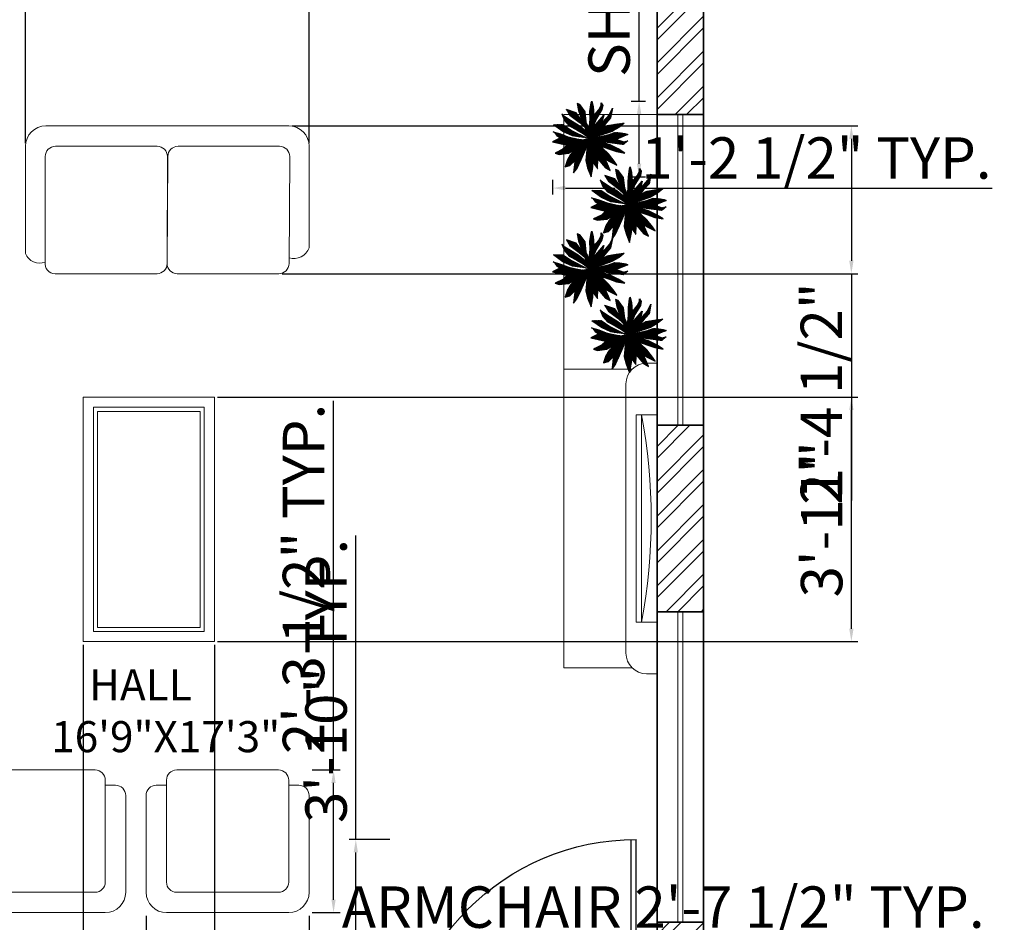
# Model space of a CAD drawing. Units: inches. Extents: x 3595 to 4516, y 2363 to 2965.
# Tile 9 of 12: x 4309 to 4499, y 2512 to 2686. Entities that reach past the tile are written whole.
import ezdxf

# ---------------------------------------------------------------- set-up
doc = ezdxf.new("R2010")
doc.units = ezdxf.units.IN
for name, color, linetype, lineweight in [('A-ANNO-DIMS', 2, 'Continuous', 18), ('A-AREA-IDEN', 7, 'Continuous', 18), ('A-DOOR', 4, 'Continuous', 25), ('A-EQPM', 8, 'Continuous', 18), ('A-FLOR-CASE', 9, 'Continuous', 18), ('A-FURN', 43, 'Continuous', 18), ('A-GLAZ', 4, 'Continuous', 18), ('A-WALL', 7, 'Continuous', 35), ('L-PLNT', 3, 'Continuous', 13), ('vfolhas', 114, 'Continuous', 5)]:
    doc.layers.add(name, color=color, linetype=linetype, lineweight=lineweight)
doc.layers.add('A-WALL-PATT', color=251, linetype='Continuous', lineweight=13, true_color=0x636466)
for name, color, linetype in [('vfolha', 72, 'Continuous'), ('vfolha2', 110, 'Continuous'), ('vfolhas2', 102, 'Continuous')]:
    doc.layers.add(name, color=color, linetype=linetype)
doc.styles.get("Standard").update_dxf_attribs({"font": 'arial.ttf'})
doc.dimstyles.new('ISO-25', dxfattribs={"dimtxt": 8, "dimasz": 2.5, "dimexe": 1.25, "dimexo": 0.625, "dimtad": 1, "dimdec": 1, "dimlunit": 3, "dimtxsty": 'Standard', "dimcen": 2.5, "dimadec": 0, "dimazin": 0, "dimtfac": 1, "dimtdec": 1, "dimtmove": 0, "dimatfit": 3, "dimfxl": 1, "dimarcsym": 0})
pattern_1 = [(45, (-2446.5133113, 50.986076), (-0.004419417382, 0.004419417382), [])]

# ---------------------------------------------------------------- blocks, each defined once
blk = doc.blocks.new('D')
for p, q in [((1, 0), (1, 46)), ((2, 0), (2, 46)), ((0, 0), (2, 0)), ((47, 0), (48, 0))]:
    blk.add_line(p, q)
at = {"ltscale": 0.5}
blk.add_arc((1, 0), 46, 0, 90, dxfattribs=at)
blk = doc.blocks.new('arbusto_PB_verde_grande')
at = {"layer": 'vfolha2'}
h = blk.add_hatch(dxfattribs=at)
h.set_pattern_fill('ANSI31', color=256, scale=0.05, style=0)
h.set_pattern_definition(pattern_1)
h.paths.add_polyline_path([(0.029, 0.357), (0, 0.09), (0.026, -0.039), (0.047, 0.062), (0.062, 0.097), (0.094, 0.266), (0.1, 0.435), (0.088, 0.613), (0.064, 0.723), (0.05, 0.685), (0.024, 0.513)])
h.paths.add_polyline_path([(0.301, 0.438), (0.142, 0.249), (0.267, 0.3)])
h.paths.add_polyline_path([(0.38, 0.228), (0.237, 0.152), (0.184, 0.094), (0.111, 0.044), (0.026, -0.039), (0.281, 0.047), (0.368, 0.078), (0.468, 0.112), (0.611, 0.194), (0.716, 0.278), (0.558, 0.259)])
h.paths.add_polyline_path([(0.561, -0.294), (0.728, -0.326), (0.59, -0.241), (0.43, -0.16), (0.026, -0.039), (0.149, -0.141), (0.188, -0.166), (0.415, -0.244)])
h.paths.add_polyline_path([(-0.274, -0.448), (-0.304, -0.726), (-0.239, -0.642), (-0.155, -0.457), (0.026, -0.039), (-0.163, -0.254)])
h.paths.add_polyline_path([(-0.52, -0.247), (-0.677, -0.326), (-0.596, -0.351), (-0.406, -0.329), (-0.21, -0.21), (0.026, -0.039), (-0.149, -0.066), (-0.315, -0.091), (-0.415, -0.15)])
h.paths.add_polyline_path([(-0.525, 0.25), (-0.709, 0.247), (-0.52, 0.109), (-0.33, 0.022), (-0.076, -0.013), (-0.042, -0.021), (-0.35, 0.131)])
h = blk.add_hatch(dxfattribs=at)
h.set_pattern_fill('ANSI31', color=256, scale=0.05, style=0)
h.set_pattern_definition(pattern_1)
h.paths.add_polyline_path([(-0.19, 0.297), (-0.086, 0.202), (-0.108, 0.25), (-0.132, 0.319), (-0.251, 0.485), (-0.45, 0.551), (-0.379, 0.438)])
h.paths.add_polyline_path([(0.079, -0.407), (0.082, -0.506), (0.173, -0.635), (0.184, -0.442), (0.149, -0.292), (0.026, -0.039), (0.035, -0.254)])
at = {"layer": 'vfolhas'}
h = blk.add_hatch(dxfattribs=at)
h.set_pattern_fill('ANSI31', color=256, scale=0.05, style=0)
h.set_pattern_definition(pattern_1)
h.paths.add_polyline_path([(-0.073, 0.507), (-0.181, 0.651), (-0.233, 0.673), (-0.207, 0.532), (-0.108, 0.25), (0.026, -0.039), (0, 0.09), (0.008, 0.162), (-0.049, 0.291)])
h.paths.add_polyline_path([(0.099, 0.419), (0.094, 0.266), (0.079, 0.188), (0.155, 0.369), (0.266, 0.551), (0.284, 0.635), (0.249, 0.688), (0.251, 0.635), (0.202, 0.544)])
h.paths.add_polyline_path([(0.123, 0.241), (0.047, 0.062), (0.026, -0.039), (0.111, 0.044), (0.184, 0.094), (0.275, 0.194), (0.322, 0.253), (0.441, 0.385), (0.476, 0.579), (0.418, 0.453), (0.289, 0.31)])
h.paths.add_polyline_path([(0.581, -0.038), (0.707, 0.015), (0.786, 0.047), (0.748, 0.065), (0.628, 0.084), (0.526, 0.09), (0.397, 0.044), (0.026, -0.039), (0.257, -0.032), (0.438, -0.035)])
h.paths.add_polyline_path([(0.52, -0.036), (0.438, -0.035), (0.257, -0.032), (0.026, -0.039), (0.18, -0.085), (0.538, -0.132), (0.695, -0.154), (0.786, -0.079), (0.704, -0.1)])
h.paths.add_polyline_path([(0.272, -0.219), (0.149, -0.141), (0.026, -0.039), (0.158, -0.31), (0.295, -0.426), (0.418, -0.492), (0.564, -0.567), (0.511, -0.485), (0.395, -0.341)])
h.paths.add_polyline_path([(-0.058, -0.476), (-0.023, -0.62), (0.047, -0.801), (0.085, -0.598), (0.079, -0.407), (0.035, -0.254), (0.026, -0.039), (-0.038, -0.26)])
h.paths.add_polyline_path([(-0.242, 0.141), (-0.111, 0.069), (0.026, -0.039), (-0.042, 0.109), (-0.21, 0.238), (-0.365, 0.331), (-0.479, 0.403), (-0.543, 0.463), (-0.49, 0.331), (-0.394, 0.222)])
h = blk.add_hatch(dxfattribs=at)
h.set_pattern_fill('ANSI31', color=256, scale=0.05, style=0)
h.set_pattern_definition(pattern_1)
h.paths.add_polyline_path([(-0.572, 0.062), (-0.715, 0.103), (-0.677, 0.081), (-0.628, 0.015), (-0.563, -0.041), (-0.265, -0.083), (-0.149, -0.066), (-0.102, -0.059), (-0.204, -0.047), (-0.403, -0.003)])
h.paths.add_polyline_path([(-0.563, -0.041), (-0.583, -0.024), (-0.73, -0.097), (-0.433, -0.168), (-0.415, -0.15), (-0.315, -0.091), (-0.265, -0.083)])
h.paths.add_polyline_path([(-0.277, -0.473), (-0.274, -0.448), (-0.163, -0.254), (0.026, -0.039), (-0.21, -0.21), (-0.267, -0.245), (-0.365, -0.357), (-0.429, -0.463), (-0.476, -0.604), (-0.379, -0.576)])
h = blk.add_hatch(dxfattribs=at)
h.set_pattern_fill('ANSI31', color=256, scale=0.05, style=0)
h.set_pattern_definition(pattern_1)
h.paths.add_polyline_path([(0.336, -0.623), (0.433, -0.673), (0.395, -0.595), (0.33, -0.445), (0.295, -0.426), (0.158, -0.31), (0.149, -0.292), (0.184, -0.442)])
at = {"layer": 'vfolha'}
for p, q in [((0.026, -0.039), (-0.149, -0.066)), ((0.026, -0.039), (-0.038, -0.26)), ((0.035, -0.254), (0.026, -0.039)), ((0.538, -0.132), (0.18, -0.085)), ((0.52, -0.036), (0.704, -0.1)), ((0.695, -0.154), (0.538, -0.132)), ((0.786, -0.079), (0.695, -0.154)), ((0.704, -0.1), (0.786, -0.079)), ((-0.267, -0.245), (-0.365, -0.357)), ((-0.038, -0.26), (-0.058, -0.476)), ((0.079, -0.407), (0.035, -0.254)), ((0.158, -0.31), (0.295, -0.426)), ((0.395, -0.341), (0.272, -0.219)), ((0.511, -0.485), (0.395, -0.341)), ((0.085, -0.598), (0.079, -0.407)), ((0.295, -0.426), (0.418, -0.492)), ((0.418, -0.492), (0.564, -0.567)), ((0.564, -0.567), (0.511, -0.485)), ((-0.023, -0.62), (0.047, -0.801)), ((0.047, -0.801), (0.085, -0.598))]:
    blk.add_line(p, q, dxfattribs=at)
at = {"layer": 'vfolha2'}
for p, q in [((0.024, 0.513), (0.05, 0.685)), ((0.05, 0.685), (0.064, 0.723)), ((0.064, 0.723), (0.088, 0.613)), ((0.088, 0.613), (0.1, 0.435)), ((-0.45, 0.551), (-0.379, 0.438)), ((-0.251, 0.485), (-0.45, 0.551)), ((-0.379, 0.438), (-0.19, 0.297)), ((-0.132, 0.319), (-0.251, 0.485)), ((0.029, 0.357), (0.024, 0.513)), ((0.1, 0.435), (0.094, 0.266)), ((0.143, 0.25), (0.301, 0.438)), ((0.301, 0.438), (0.266, 0.297)), ((-0.709, 0.247), (-0.525, 0.25)), ((-0.52, 0.109), (-0.709, 0.247)), ((-0.525, 0.25), (-0.35, 0.131)), ((-0.19, 0.297), (-0.082, 0.199)), ((0, 0.09), (0.029, 0.357)), ((0.237, 0.152), (0.38, 0.228)), ((0.38, 0.228), (0.558, 0.259)), ((0.558, 0.259), (0.716, 0.278)), ((0.716, 0.278), (0.611, 0.194)), ((-0.33, 0.022), (-0.52, 0.109)), ((-0.35, 0.131), (-0.042, -0.021)), ((-0.076, -0.013), (-0.33, 0.022)), ((0.026, -0.039), (0, 0.09)), ((0.281, 0.047), (0.026, -0.039)), ((0.368, 0.078), (0.281, 0.047)), ((0.611, 0.194), (0.468, 0.112)), ((-0.415, -0.15), (-0.52, -0.247)), ((-0.315, -0.091), (-0.415, -0.15)), ((-0.149, -0.066), (-0.315, -0.091)), ((-0.21, -0.21), (0.026, -0.039)), ((0.026, -0.039), (-0.163, -0.254)), ((-0.155, -0.457), (0.026, -0.039)), ((0.43, -0.16), (0.026, -0.039)), ((0.026, -0.039), (0.158, -0.31)), ((0.188, -0.166), (0.415, -0.244)), ((0.59, -0.241), (0.43, -0.16)), ((-0.52, -0.247), (-0.677, -0.326)), ((-0.677, -0.326), (-0.596, -0.351)), ((-0.596, -0.351), (-0.406, -0.329)), ((-0.406, -0.329), (-0.21, -0.21)), ((-0.163, -0.254), (-0.274, -0.448)), ((0.184, -0.442), (0.149, -0.292)), ((0.415, -0.244), (0.561, -0.294)), ((0.561, -0.294), (0.728, -0.326)), ((0.728, -0.326), (0.59, -0.241)), ((-0.274, -0.448), (-0.304, -0.726)), ((0.082, -0.506), (0.173, -0.635)), ((0.173, -0.635), (0.184, -0.442)), ((-0.304, -0.726), (-0.239, -0.642))]:
    blk.add_line(p, q, dxfattribs=at)
at = {"layer": 'vfolhas2'}
for p, q in [((-0.233, 0.673), (-0.207, 0.532)), ((-0.181, 0.651), (-0.233, 0.673)), ((-0.073, 0.507), (-0.181, 0.651)), ((0.202, 0.544), (0.251, 0.635)), ((0.251, 0.635), (0.249, 0.688)), ((0.249, 0.688), (0.284, 0.635)), ((0.284, 0.635), (0.266, 0.551)), ((-0.543, 0.463), (-0.49, 0.331)), ((-0.479, 0.403), (-0.543, 0.463)), ((-0.365, 0.331), (-0.479, 0.403)), ((-0.207, 0.532), (-0.108, 0.25)), ((-0.049, 0.291), (-0.073, 0.507)), ((0.099, 0.419), (0.202, 0.544)), ((0.266, 0.551), (0.155, 0.369)), ((0.289, 0.31), (0.418, 0.453)), ((0.418, 0.453), (0.476, 0.579)), ((0.476, 0.579), (0.441, 0.385)), ((-0.49, 0.331), (-0.394, 0.222)), ((-0.394, 0.222), (-0.242, 0.141)), ((-0.21, 0.238), (-0.365, 0.331)), ((-0.042, 0.109), (-0.21, 0.238)), ((-0.108, 0.25), (0.026, -0.039)), ((0.008, 0.162), (-0.049, 0.291)), ((0.047, 0.062), (0.123, 0.241)), ((0.094, 0.266), (0.062, 0.097)), ((0.155, 0.369), (0.078, 0.186)), ((0.123, 0.241), (0.289, 0.31)), ((0.322, 0.253), (0.275, 0.194)), ((0.441, 0.385), (0.322, 0.253)), ((-0.677, 0.081), (-0.715, 0.103)), ((-0.715, 0.103), (-0.572, 0.062)), ((-0.628, 0.015), (-0.677, 0.081)), ((-0.563, -0.041), (-0.628, 0.015)), ((-0.572, 0.062), (-0.403, -0.003)), ((-0.242, 0.141), (-0.111, 0.069)), ((-0.111, 0.069), (0.026, -0.039)), ((0.026, -0.039), (0.047, 0.062)), ((0.026, -0.039), (0.397, 0.044)), ((0.111, 0.044), (0.026, -0.039)), ((0.184, 0.094), (0.111, 0.044)), ((0.275, 0.194), (0.184, 0.094)), ((0.468, 0.112), (0.368, 0.078)), ((0.397, 0.044), (0.526, 0.09)), ((0.526, 0.09), (0.628, 0.084)), ((0.707, 0.015), (0.581, -0.038)), ((0.628, 0.084), (0.748, 0.065)), ((0.786, 0.047), (0.707, 0.015)), ((0.748, 0.065), (0.786, 0.047)), ((-0.583, -0.024), (-0.73, -0.097)), ((-0.73, -0.097), (-0.433, -0.168)), ((-0.265, -0.083), (-0.563, -0.041)), ((-0.403, -0.003), (-0.204, -0.047)), ((-0.204, -0.047), (-0.098, -0.059)), ((0.026, -0.039), (-0.076, -0.013)), ((0.257, -0.032), (0.026, -0.039)), ((0.149, -0.141), (0.026, -0.039)), ((0.272, -0.219), (0.149, -0.141)), ((0.438, -0.035), (0.257, -0.032)), ((0.581, -0.038), (0.438, -0.035)), ((-0.365, -0.357), (-0.429, -0.463)), ((-0.429, -0.463), (-0.476, -0.604)), ((-0.476, -0.604), (-0.379, -0.576)), ((-0.379, -0.576), (-0.277, -0.473)), ((-0.239, -0.642), (-0.155, -0.457)), ((-0.058, -0.476), (-0.023, -0.62)), ((0.184, -0.442), (0.336, -0.623)), ((0.395, -0.595), (0.329, -0.442)), ((0.433, -0.673), (0.395, -0.595)), ((0.336, -0.623), (0.433, -0.673))]:
    blk.add_line(p, q, dxfattribs=at)
blk = doc.blocks.new('WIN-GLAZING-60IN')
for p, q in [((0, 60), (0, 0)), ((1, 60), (1, 0))]:
    blk.add_line(p, q)
blk = doc.blocks.new('LOUNGE-ARMCHAIR')
for p, q in [((5.91, 27.56), (25.59, 27.56)), ((3.94, 5.91), (3.94, 25.59)), ((27.56, 25.59), (27.56, 5.91)), ((1.97, 24.61), (3.94, 24.61)), ((27.56, 24.61), (29.53, 24.61)), ((0, 3.94), (0, 22.64)), ((31.5, 22.64), (31.5, 3.94)), ((25.59, 3.94), (5.91, 3.94)), ((27.56, 0), (3.94, 0))]:
    blk.add_line(p, q)
for centre, radius, start, end in [((5.91, 25.59), 1.97, 90, 180), ((25.59, 25.59), 1.97, 360, 90), ((1.97, 22.64), 1.97, 90, 180), ((29.53, 22.64), 1.97, 360, 90), ((5.91, 5.91), 1.97, 180, 270), ((25.59, 5.91), 1.97, 270, 0), ((3.94, 3.94), 3.94, 180, 270), ((27.56, 3.94), 3.94, 270, 0)]:
    blk.add_arc(centre, radius, start, end)
blk = doc.blocks.new('*D114')
at = {"layer": 'A-ANNO-DIMS', "color": 0, "lineweight": -2, "transparency": 16777216}
for p, q in [((4374.04, 2527.54), (4374.04, 2586.27)), ((4380.62, 2527.54), (4372.79, 2527.54)), ((4374.04, 2484.04), (4374.04, 2525.04)), ((4380.62, 2481.54), (4372.79, 2481.54))]:
    blk.add_line(p, q, dxfattribs=at)
at = {"layer": 'A-ANNO-DIMS', "color": 0, "transparency": 16777216}
for points in [[(4373.63, 2525.04), (4374.46, 2525.04), (4374.04, 2527.54)], [(4373.63, 2484.04), (4374.46, 2484.04), (4374.04, 2481.54)]]:
    blk.add_solid(points, dxfattribs=at)
at = {"layer": 'Defpoints', "color": 0, "transparency": 16777216}
for p in [(4374.04, 2527.54), (4381.24, 2527.54), (4381.24, 2481.54)]:
    blk.add_point(p, dxfattribs=at)
at = {"layer": 'A-ANNO-DIMS', "color": 0, "transparency": 16777216, "insert": (4369.33, 2558.16), "char_height": 8, "attachment_point": 5, "rotation": 90}
blk.add_mtext('3\'-10" TYP.', dxfattribs=at)
blk = doc.blocks.new('*D139')
at = {"layer": 'A-ANNO-DIMS', "color": 0, "lineweight": -2, "transparency": 16777216}
for p, q in [((4333.52, 2512.78), (4333.52, 2507.43)), ((4365.01, 2512.78), (4365.01, 2507.43)), ((4336.02, 2508.68), (4362.51, 2508.68)), ((4365.01, 2508.68), (4499.34, 2508.68))]:
    blk.add_line(p, q, dxfattribs=at)
at = {"layer": 'A-ANNO-DIMS', "color": 0, "transparency": 16777216}
for points in [[(4336.02, 2509.1), (4336.02, 2508.27), (4333.52, 2508.68)], [(4362.51, 2509.1), (4362.51, 2508.27), (4365.01, 2508.68)]]:
    blk.add_solid(points, dxfattribs=at)
at = {"layer": 'Defpoints', "color": 0, "transparency": 16777216}
for p in [(4333.52, 2513.41), (4365.01, 2513.41), (4365.01, 2508.68)]:
    blk.add_point(p, dxfattribs=at)
at = {"layer": 'A-ANNO-DIMS', "color": 0, "transparency": 16777216, "insert": (4433.43, 2513.44), "char_height": 8, "attachment_point": 5}
blk.add_mtext('ARMCHAIR 2\'-7 1/2" TYP.', dxfattribs=at)
blk = doc.blocks.new('*D140')
at = {"layer": 'A-ANNO-DIMS', "color": 0, "lineweight": -2, "transparency": 16777216}
for p, q in [((4369.74, 2540.97), (4369.74, 2612.26)), ((4365.64, 2540.97), (4370.99, 2540.97)), ((4369.74, 2515.91), (4369.74, 2538.47)), ((4365.64, 2513.41), (4370.99, 2513.41))]:
    blk.add_line(p, q, dxfattribs=at)
at = {"layer": 'A-ANNO-DIMS', "color": 0, "transparency": 16777216}
for points in [[(4369.32, 2538.47), (4370.15, 2538.47), (4369.74, 2540.97)], [(4369.32, 2515.91), (4370.15, 2515.91), (4369.74, 2513.41)]]:
    blk.add_solid(points, dxfattribs=at)
at = {"layer": 'Defpoints', "color": 0, "transparency": 16777216}
for p in [(4365.01, 2540.97), (4369.74, 2540.97), (4365.01, 2513.41)]:
    blk.add_point(p, dxfattribs=at)
at = {"layer": 'A-ANNO-DIMS', "color": 0, "transparency": 16777216, "insert": (4364.97, 2577.86), "char_height": 8, "attachment_point": 5, "rotation": 90}
blk.add_mtext('2\'-3 1/2" TYP.', dxfattribs=at)
blk = doc.blocks.new('*D143')
at = {"layer": 'A-ANNO-DIMS', "color": 0, "lineweight": -2, "transparency": 16777216}
for p, q in [((4428.78, 2670.16), (4428.78, 2783.51)), ((4427.22, 2670.16), (4430.03, 2670.16)), ((4428.78, 2658.05), (4428.78, 2667.66)), ((4427.22, 2655.55), (4430.03, 2655.55))]:
    blk.add_line(p, q, dxfattribs=at)
at = {"layer": 'A-ANNO-DIMS', "color": 0, "transparency": 16777216}
for points in [[(4428.37, 2667.66), (4429.2, 2667.66), (4428.78, 2670.16)], [(4428.37, 2658.05), (4429.2, 2658.05), (4428.78, 2655.55)]]:
    blk.add_solid(points, dxfattribs=at)
at = {"layer": 'Defpoints', "color": 0, "transparency": 16777216}
for p in [(4426.59, 2670.16), (4428.78, 2670.16), (4426.59, 2655.55)]:
    blk.add_point(p, dxfattribs=at)
at = {"layer": 'A-ANNO-DIMS', "color": 0, "transparency": 16777216, "insert": (4424.02, 2728.08), "char_height": 8, "attachment_point": 5, "rotation": 90}
blk.add_mtext('SHRUB 1\'-2 1/2" TYP.', dxfattribs=at)
blk = doc.blocks.new('*D144')
at = {"layer": 'A-ANNO-DIMS', "color": 0, "lineweight": -2, "transparency": 16777216}
for p, q in [((4412.05, 2654.92), (4412.05, 2652.1)), ((4426.59, 2654.92), (4426.59, 2652.1)), ((4414.55, 2653.35), (4424.09, 2653.35)), ((4426.59, 2653.35), (4496.99, 2653.35))]:
    blk.add_line(p, q, dxfattribs=at)
at = {"layer": 'A-ANNO-DIMS', "color": 0, "transparency": 16777216}
for points in [[(4414.55, 2653.77), (4414.55, 2652.94), (4412.05, 2653.35)], [(4424.09, 2653.77), (4424.09, 2652.94), (4426.59, 2653.35)]]:
    blk.add_solid(points, dxfattribs=at)
at = {"layer": 'Defpoints', "color": 0, "transparency": 16777216}
for p in [(4412.05, 2655.55), (4426.59, 2655.55), (4426.59, 2653.35)]:
    blk.add_point(p, dxfattribs=at)
at = {"layer": 'A-ANNO-DIMS', "color": 0, "transparency": 16777216, "insert": (4463.04, 2658.12), "char_height": 8, "attachment_point": 5}
blk.add_mtext('1\'-2 1/2" TYP.', dxfattribs=at)
blk = doc.blocks.new('*D161')
at = {"layer": 'A-ANNO-DIMS', "color": 0, "lineweight": -2, "transparency": 16777216}
for p, q in [((4321.38, 2565.12), (4321.38, 2369.24)), ((4346.72, 2565.12), (4346.72, 2369.24)), ((4323.88, 2370.49), (4344.22, 2370.49)), ((4346.72, 2370.49), (4390.51, 2370.49))]:
    blk.add_line(p, q, dxfattribs=at)
at = {"layer": 'A-ANNO-DIMS', "color": 0, "transparency": 16777216}
for points in [[(4323.88, 2370.91), (4323.88, 2370.08), (4321.38, 2370.49)], [(4344.22, 2370.91), (4344.22, 2370.08), (4346.72, 2370.49)]]:
    blk.add_solid(points, dxfattribs=at)
at = {"layer": 'Defpoints', "color": 0, "transparency": 16777216}
for p in [(4321.38, 2565.75), (4346.72, 2565.75), (4346.72, 2370.49)]:
    blk.add_point(p, dxfattribs=at)
at = {"layer": 'A-ANNO-DIMS', "color": 0, "transparency": 16777216, "insert": (4369.86, 2375.26), "char_height": 8, "attachment_point": 5}
blk.add_mtext('2\'-1 1/2"', dxfattribs=at)
blk = doc.blocks.new('*D162')
at = {"layer": 'A-ANNO-DIMS', "color": 0, "lineweight": -2, "transparency": 16777216}
for p, q in [((4347.34, 2612.99), (4471.04, 2612.99)), ((4469.79, 2568.25), (4469.79, 2610.49)), ((4347.34, 2565.75), (4471.04, 2565.75))]:
    blk.add_line(p, q, dxfattribs=at)
at = {"layer": 'A-ANNO-DIMS', "color": 0, "transparency": 16777216}
for points in [[(4469.38, 2610.49), (4470.21, 2610.49), (4469.79, 2612.99)], [(4469.38, 2568.25), (4470.21, 2568.25), (4469.79, 2565.75)]]:
    blk.add_solid(points, dxfattribs=at)
at = {"layer": 'Defpoints', "color": 0, "transparency": 16777216}
for p in [(4346.72, 2612.99), (4469.79, 2612.99), (4346.72, 2565.75)]:
    blk.add_point(p, dxfattribs=at)
at = {"layer": 'A-ANNO-DIMS', "color": 0, "transparency": 16777216, "insert": (4465.08, 2589.37), "char_height": 8, "attachment_point": 5, "rotation": 90}
blk.add_mtext('3\'-11"', dxfattribs=at)
blk = doc.blocks.new('*D163')
at = {"layer": 'A-ANNO-DIMS', "color": 0, "lineweight": -2, "transparency": 16777216}
for p, q in [((4267.47, 2626.41), (4267.47, 2932.84)), ((4295.03, 2624.44), (4295.03, 2932.84)), ((4269.97, 2931.59), (4292.53, 2931.59)), ((4295.03, 2931.59), (4338.82, 2931.59))]:
    blk.add_line(p, q, dxfattribs=at)
at = {"layer": 'A-ANNO-DIMS', "color": 0, "transparency": 16777216}
for points in [[(4269.97, 2932.01), (4269.97, 2931.18), (4267.47, 2931.59)], [(4292.53, 2932.01), (4292.53, 2931.18), (4295.03, 2931.59)]]:
    blk.add_solid(points, dxfattribs=at)
at = {"layer": 'Defpoints', "color": 0, "transparency": 16777216}
for p in [(4295.03, 2931.59), (4267.47, 2625.78), (4295.03, 2623.82)]:
    blk.add_point(p, dxfattribs=at)
at = {"layer": 'A-ANNO-DIMS', "color": 0, "transparency": 16777216, "insert": (4318.18, 2936.36), "char_height": 8, "attachment_point": 5}
blk.add_mtext('2\'-3 1/2"', dxfattribs=at)
blk = doc.blocks.new('*D165')
at = {"layer": 'A-ANNO-DIMS', "color": 0, "lineweight": -2, "transparency": 16777216}
for p, q in [((4310.22, 2662.04), (4310.22, 2932.84)), ((4365.03, 2662.04), (4365.03, 2932.84)), ((4312.72, 2931.59), (4362.53, 2931.59))]:
    blk.add_line(p, q, dxfattribs=at)
at = {"layer": 'A-ANNO-DIMS', "color": 0, "transparency": 16777216}
for points in [[(4312.72, 2932.01), (4312.72, 2931.18), (4310.22, 2931.59)], [(4362.53, 2932.01), (4362.53, 2931.18), (4365.03, 2931.59)]]:
    blk.add_solid(points, dxfattribs=at)
at = {"layer": 'Defpoints', "color": 0, "transparency": 16777216}
for p in [(4365.03, 2931.59), (4310.22, 2661.42), (4365.03, 2661.42)]:
    blk.add_point(p, dxfattribs=at)
at = {"layer": 'A-ANNO-DIMS', "color": 0, "transparency": 16777216, "insert": (4337.62, 2936.22), "char_height": 8, "attachment_point": 5}
blk.add_mtext('4\'-7"', dxfattribs=at)
blk = doc.blocks.new('*D166')
at = {"layer": 'A-ANNO-DIMS', "color": 0, "lineweight": -2, "transparency": 16777216}
for p, q in [((4361.72, 2665.35), (4471.04, 2665.35)), ((4469.79, 2662.85), (4469.79, 2639.31)), ((4359.8, 2636.81), (4471.04, 2636.81)), ((4469.79, 2636.81), (4469.79, 2593.02))]:
    blk.add_line(p, q, dxfattribs=at)
at = {"layer": 'A-ANNO-DIMS', "color": 0, "transparency": 16777216}
for points in [[(4469.38, 2662.85), (4470.21, 2662.85), (4469.79, 2665.35)], [(4469.38, 2639.31), (4470.21, 2639.31), (4469.79, 2636.81)]]:
    blk.add_solid(points, dxfattribs=at)
at = {"layer": 'Defpoints', "color": 0, "transparency": 16777216}
for p in [(4361.09, 2665.35), (4359.17, 2636.81), (4469.79, 2636.81)]:
    blk.add_point(p, dxfattribs=at)
at = {"layer": 'A-ANNO-DIMS', "color": 0, "transparency": 16777216, "insert": (4465.03, 2613.66), "char_height": 8, "attachment_point": 5, "rotation": 90}
blk.add_mtext('2\'-4 1/2"', dxfattribs=at)

msp = doc.modelspace()

# ---------------------------------------------------------------- hatches: boundary and pattern name
at = {"layer": 'A-WALL-PATT'}
h = msp.add_hatch(dxfattribs=at)
h.set_pattern_fill('ANSI32', color=256, scale=0.5)
h.set_pattern_definition([(45, (441.351, 0), (-3.367596, 3.367596), []), (45, (443.596, 0), (-3.367596, 3.367596), [])])
h.paths.add_polyline_path([(4081.24, 2756.04), (4090.24, 2756.04), (4090.24, 2894.04), (4168.24, 2894.04), (4168.24, 2903.04), (4081.24, 2903.04)])
h.paths.add_polyline_path([(4216.24, 2903.04), (4216.24, 2894.04), (4222.24, 2894.04), (4222.24, 2792.04), (4231.24, 2792.04), (4231.24, 2894.04), (4241.74, 2894.04), (4241.74, 2903.04)])
h.paths.add_polyline_path([(4324.24, 2894.04), (4324.24, 2903.04), (4277.74, 2903.04), (4277.74, 2894.04), (4288.24, 2894.04), (4288.24, 2798.04), (4261.24, 2798.04), (4261.24, 2792.04), (4288.24, 2792.04), (4288.24, 2756.04), (4222.24, 2756.04), (4222.24, 2702.04), (4219.24, 2702.04), (4219.24, 2693.04), (4241.74, 2693.04), (4241.74, 2702.04), (4231.24, 2702.04), (4231.24, 2750.04), (4288.24, 2750.04), (4288.24, 2702.04), (4277.74, 2702.04), (4277.74, 2693.04), (4393.24, 2693.04), (4393.24, 2702.04), (4294.24, 2702.04), (4294.24, 2840.04), (4396.24, 2840.04), (4396.24, 2846.04), (4294.24, 2846.04), (4294.24, 2894.04)])
h.paths.add_polyline_path([(4390.24, 2894.04), (4390.24, 2876.04), (4396.24, 2876.04), (4396.24, 2894.04), (4432.24, 2894.04), (4432.24, 2795.04), (4441.24, 2795.04), (4441.24, 2903.04), (4360.24, 2903.04), (4360.24, 2894.04)])
h.paths.add_polyline_path([(4090.24, 2693.04), (4183.24, 2693.04), (4183.24, 2702.04), (4090.24, 2702.04), (4090.24, 2708.04), (4081.24, 2708.04), (4081.24, 2673.54), (4090.24, 2673.54)])
h.paths.add_polyline_path([(4090.24, 2600.04), (4183.24, 2600.04), (4183.24, 2606.04), (4090.24, 2606.04), (4090.24, 2625.54), (4081.24, 2625.54), (4081.24, 2561.04), (4090.24, 2561.04)])
h.paths.add_polyline_path([(4081.24, 2399.04), (4231.24, 2399.04), (4231.24, 2405.04), (4090.24, 2405.04), (4090.24, 2477.04), (4180.24, 2477.04), (4180.24, 2486.04), (4090.24, 2486.04), (4090.24, 2525.04), (4081.24, 2525.04)])
h.paths.add_polyline_path([(4231.24, 2486.04), (4231.24, 2606.04), (4219.24, 2606.04), (4219.24, 2600.04), (4222.24, 2600.04), (4222.24, 2486.04), (4216.24, 2486.04), (4216.24, 2477.04), (4273.24, 2477.04), (4273.24, 2486.04)])
h.paths.add_polyline_path([(4339.24, 2486.04), (4339.24, 2477.04), (4381.24, 2477.04), (4381.24, 2486.04)])
h.paths.add_polyline_path([(4432.24, 2486.04), (4429.24, 2486.04), (4429.24, 2477.04), (4441.24, 2477.04), (4441.24, 2511.54), (4432.24, 2511.54)])
h.paths.add_polyline_path([(4432.24, 2571.54), (4441.24, 2571.54), (4441.24, 2607.54), (4432.24, 2607.54)])
h.paths.add_polyline_path([(4441.24, 2747.04), (4432.24, 2747.04), (4432.24, 2702.04), (4429.24, 2702.04), (4429.24, 2693.04), (4432.24, 2693.04), (4432.24, 2667.54), (4441.24, 2667.54)])

# ---------------------------------------------------------------- linework, layer by layer
at = {"layer": 'A-EQPM'}
for p, q in [((4432.24, 2609.54), (4428.24, 2609.54)), ((4428.24, 2569.54), (4428.24, 2609.54)), ((4429.24, 2569.54), (4429.24, 2609.54)), ((4432.24, 2569.54), (4428.24, 2569.54))]:
    msp.add_line(p, q, dxfattribs=at)
msp.add_arc((4324.21, 2589.54), 106.92, 349.2189, 10.7811, dxfattribs=at)
at = {"layer": 'A-FLOR-CASE'}
for p, q in [((4414.24, 2667.54), (4414.24, 2560.72)), ((4432.24, 2667.54), (4414.24, 2667.54)), ((4427.42, 2618.37), (4414.24, 2618.37)), ((4432.24, 2619.54), (4430.24, 2619.54)), ((4426.24, 2615.54), (4426.24, 2563.54)), ((4427.42, 2560.72), (4414.24, 2560.72)), ((4432.24, 2559.54), (4430.24, 2559.54))]:
    msp.add_line(p, q, dxfattribs=at)
for centre, start, end in [((4430.24, 2615.54), 90, 180), ((4430.24, 2563.54), 180, 270)]:
    msp.add_arc(centre, 4, start, end, dxfattribs=at)
at = {"layer": 'A-FURN'}
for p, q in [((4314.16, 2665.35), (4361.09, 2665.35)), ((4310.22, 2640.71), (4310.22, 2661.42)), ((4316, 2661.42), (4335.68, 2661.42)), ((4359.3, 2661.42), (4339.69, 2661.42)), ((4365.03, 2661.42), (4365.03, 2641.82)), ((4314.03, 2639.07), (4314.03, 2659.45)), ((4337.65, 2659.45), (4337.58, 2638.78)), ((4337.72, 2659.45), (4337.58, 2638.78)), ((4361.14, 2638.77), (4361.27, 2659.45)), ((4335.68, 2636.81), (4315.95, 2636.81)), ((4339.55, 2636.81), (4359.17, 2636.81))]:
    msp.add_line(p, q, dxfattribs=at)
for points in [[(4346.72, 2612.99), (4346.72, 2565.75), (4321.38, 2565.75), (4321.38, 2612.99)], [(4344.75, 2611.02), (4344.75, 2567.71), (4323.35, 2567.71), (4323.35, 2611.02)], [(4343.96, 2610.23), (4343.96, 2568.5), (4324.13, 2568.5), (4324.13, 2610.23)]]:
    msp.add_lwpolyline(points, close=True, dxfattribs=at)
for centre, radius, start, end in [((4314.16, 2661.42), 3.94, 90, 180), ((4361.09, 2661.42), 3.94, 0, 90), ((4316, 2659.45), 1.97, 90, 180), ((4335.68, 2659.45), 1.97, 360, 90), ((4339.69, 2659.45), 1.97, 90, 180), ((4359.3, 2659.45), 1.97, 360, 90), ((4312.93, 2641.77), 2.91, 201.3314, 292.0931), ((4362.03, 2642.92), 3.19, 253.8468, 339.9238), ((4315.94, 2638.75), 1.94, 170.2828, 270.3826), ((4335.62, 2638.78), 1.97, 270, 0), ((4339.55, 2638.78), 1.97, 180, 270), ((4359.17, 2638.78), 1.97, 270, 0)]:
    msp.add_arc(centre, radius, start, end, dxfattribs=at)
at = {"layer": 'A-WALL'}
for p, q in [((4432.24, 2693.04), (4432.24, 2486.04)), ((4441.24, 2667.54), (4432.24, 2667.54)), ((4441.24, 2607.54), (4432.24, 2607.54)), ((4441.24, 2571.54), (4432.24, 2571.54)), ((4441.24, 2511.54), (4432.24, 2511.54))]:
    msp.add_line(p, q, dxfattribs=at)
msp.add_lwpolyline([(4231.24, 2399.04), (4081.24, 2399.04), (4081.24, 2903.04), (4441.24, 2903.04), (4441.24, 2477.04)], dxfattribs=at)

# ---------------------------------------------------------------- block references
at = {"layer": 'A-DOOR', "xscale": -1}
msp.add_blockref('D', (4429.24, 2481.54), dxfattribs=at)
at = {"layer": 'A-FURN'}
for p in [(4298.08, 2513.41), (4333.52, 2513.41)]:
    msp.add_blockref('LOUNGE-ARMCHAIR', p, dxfattribs=at)
at = {"layer": 'A-GLAZ', "rotation": 180}
for p in [(4437.24, 2667.54), (4437.24, 2571.54)]:
    msp.add_blockref('WIN-GLAZING-60IN', p, dxfattribs=at)
at = {"layer": 'L-PLNT', "xscale": 9.590574595713443, "yscale": 9.590574595713443, "zscale": 9.590574595713443}
for p in [(4419.05, 2663.23), (4426.47, 2650.51), (4419.05, 2638.09), (4426.47, 2625.37)]:
    msp.add_blockref('arbusto_PB_verde_grande', p, dxfattribs=at)

# ---------------------------------------------------------------- texts
at = {"layer": 'A-AREA-IDEN', "insert": (4315.18, 2560.4), "char_height": 6, "attachment_point": 1}
msp.add_mtext_dynamic_manual_height_columns('{\\fTimes New Roman|b0|i0|c0|p18;    HALL\\P16\'9"X17\'3"}', width=67.3508, gutter_width=12.5, heights=[0], dxfattribs=at)

# ---------------------------------------------------------------- dimensions: what is measured, and where the dimension line sits
at = {"layer": 'A-ANNO-DIMS'}
for base, p1, p2, picture, middle in [((4295.03, 2931.59), (4267.47, 2625.78), (4295.03, 2623.82), '*D163', (4318.18, 2936.36)), ((4365.03, 2931.59), (4310.22, 2661.42), (4365.03, 2661.42), '*D165', (4337.62, 2936.22)), ((4346.72, 2370.49), (4321.38, 2565.75), (4346.72, 2565.75), '*D161', (4369.86, 2375.26))]:
    dim = msp.add_linear_dim(base=base, p1=p1, p2=p2, dimstyle='ISO-25', override={"dimdec": 1, "dimlfac": 1, "dimrnd": 0, "dimzin": 1, "dimdsep": 46, "dimlunit": 4, "dimfrac": 2}, dxfattribs=at)
    dim.commit()
    dim.dimension.update_dxf_attribs({"geometry": picture, "text_midpoint": middle})
for base, p1, p2, text, picture, middle in [((4428.78, 2670.16), (4426.59, 2655.55), (4426.59, 2670.16), 'SHRUB <> TYP.', '*D143', (4424.02, 2728.08)), ((4369.74, 2540.97), (4365.01, 2513.41), (4365.01, 2540.97), '<> TYP.', '*D140', (4364.97, 2577.86)), ((4374.04, 2527.54), (4381.24, 2481.54), (4381.24, 2527.54), '<> TYP.', '*D114', (4369.33, 2558.16))]:
    dim = msp.add_linear_dim(base=base, p1=p1, p2=p2, angle=90, text=text, dimstyle='ISO-25', override={"dimdec": 1, "dimlfac": 1, "dimrnd": 0, "dimzin": 1, "dimdsep": 46, "dimlunit": 4, "dimfrac": 2}, dxfattribs=at)
    dim.commit()
    dim.dimension.update_dxf_attribs({"geometry": picture, "text_midpoint": middle})
for base, p1, p2, text, picture, middle in [((4426.59, 2653.35), (4412.05, 2655.55), (4426.59, 2655.55), '<> TYP.', '*D144', (4463.04, 2658.12)), ((4365.01, 2508.68), (4333.52, 2513.41), (4365.01, 2513.41), 'ARMCHAIR <> TYP.', '*D139', (4433.43, 2513.44))]:
    dim = msp.add_linear_dim(base=base, p1=p1, p2=p2, text=text, dimstyle='ISO-25', override={"dimdec": 1, "dimlfac": 1, "dimrnd": 0, "dimzin": 1, "dimdsep": 46, "dimlunit": 4, "dimfrac": 2}, dxfattribs=at)
    dim.commit()
    dim.dimension.update_dxf_attribs({"geometry": picture, "text_midpoint": middle})
for base, p1, p2, picture, middle in [((4469.79, 2636.81), (4361.09, 2665.35), (4359.17, 2636.81), '*D166', (4465.03, 2613.66)), ((4469.79, 2612.99), (4346.72, 2565.75), (4346.72, 2612.99), '*D162', (4465.08, 2589.37))]:
    dim = msp.add_linear_dim(base=base, p1=p1, p2=p2, angle=90, dimstyle='ISO-25', override={"dimdec": 1, "dimlfac": 1, "dimrnd": 0, "dimzin": 1, "dimdsep": 46, "dimlunit": 4, "dimfrac": 2}, dxfattribs=at)
    dim.commit()
    dim.dimension.update_dxf_attribs({"geometry": picture, "text_midpoint": middle})

doc.saveas('drawing.dxf')
